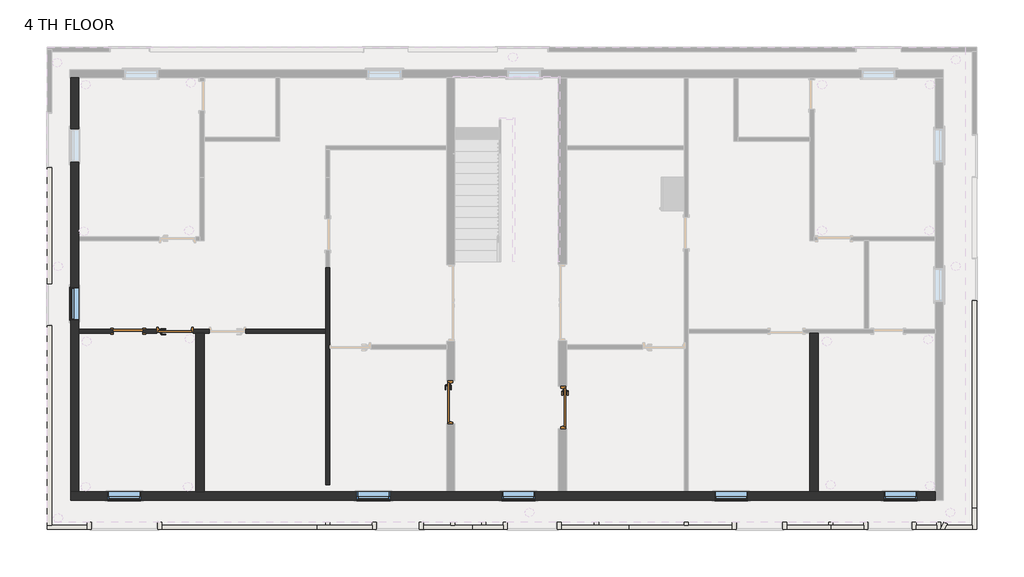
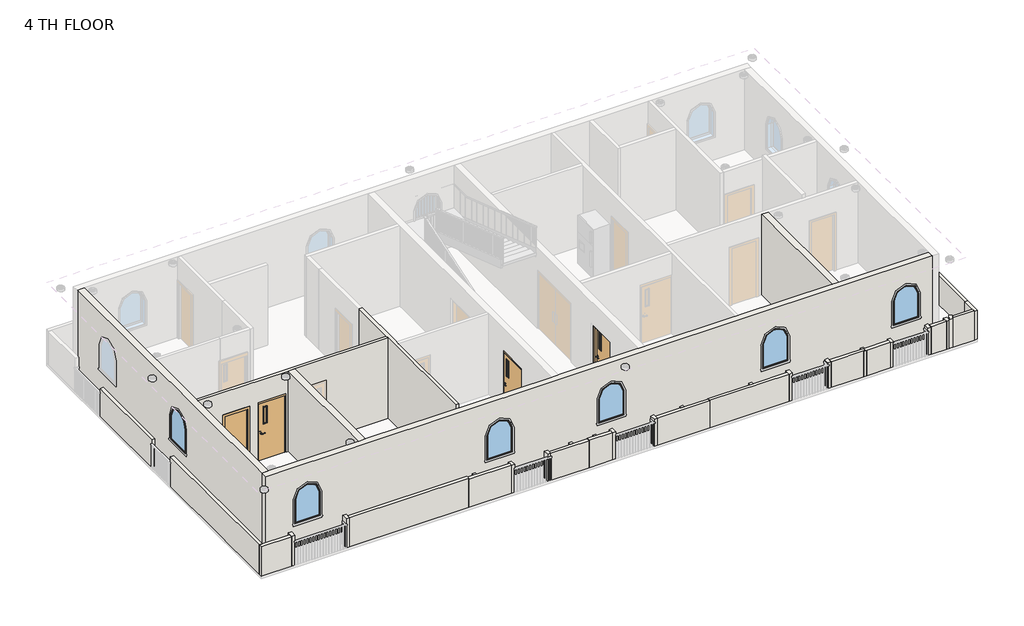
# One storey, part 1 of 7: 39 walls, 6 windows, 4 doors.
# Revit data of these elements (continued)
# Element 4 (IfcDoor, "Single-Flush : 2'8\"x 7'") (continued)
#   Phase Created = New Construction
#   Materials on its faces: "Door - Frame", "Door - Panel"
# Elements 5, 6 (IfcWall, "Generic - 4.5\"")
#   Top Offset = -0' - 6"
#   Base Offset = 0' - 0"
#   wall height = 10' - 0"
#   Phase Created = New Construction
#   Base Constraint = 4 TH FLOOR
#   Top Constraint = 5TH FLOOR
#   Materials on its faces: "Default Wall"
# Element 7 (IfcWall, "Generic - 4.5\"")
#   Top Offset = -6' - 10.1834"
#   Base Offset = 0' - 0"
#   wall height = 3' - 7.8166"
#   Phase Created = New Construction
#   Base Constraint = 4 TH FLOOR
#   Top Constraint = 5TH FLOOR
#   Materials on its faces: "Default Wall"
# Element 8 (IfcWall, "Generic - 4.5\"")
#   Top Offset = 0' - 0"
#   Base Offset = 0' - 0"
#   Unconnected Height = 3' - 8.64293"
#   wall height = 3' - 8.64293"
#   Phase Created = New Construction
#   Base Constraint = 4 TH FLOOR
#   Materials on its faces: "Default Wall"
# Element 9 (IfcWall, "Generic - 4.5\"")
#   Top Offset = -6' - 10.57009"
#   Base Offset = 0' - 0"
#   wall height = 3' - 7.42991"
#   Phase Created = New Construction
#   Base Constraint = 4 TH FLOOR
#   Top Constraint = 5TH FLOOR
#   Materials on its faces: "Default Wall"
# Element 10 (IfcWall, "Generic - 4.5\"")
#   Top Offset = -6' - 11.10495"
#   Base Offset = 0' - 0"
#   wall height = 3' - 6.89505"
#   Phase Created = New Construction
#   Base Constraint = 4 TH FLOOR
#   Top Constraint = 5TH FLOOR
#   Materials on its faces: "Default Wall"
# Element 11 (IfcWall, "Generic - 4.5\"")
#   Top Offset = -6' - 11.01332"
#   Base Offset = 0' - 0"
#   wall height = 3' - 6.98668"
#   Phase Created = New Construction
#   Base Constraint = 4 TH FLOOR
#   Top Constraint = 5TH FLOOR
#   Materials on its faces: "Default Wall"
# Element 12 (IfcWall, "Generic - 4.5\"")
#   Top Offset = -7' - 0.14651"
#   Base Offset = 0' - 0"
#   wall height = 3' - 5.85349"
#   Phase Created = New Construction
#   Base Constraint = 4 TH FLOOR
#   Top Constraint = 5TH FLOOR
#   Materials on its faces: "Default Wall"
# Element 13 (IfcWall, "Generic - 4.5\"")
#   Top Offset = -6' - 11.98199"
#   Base Offset = 0' - 0"
#   wall height = 3' - 6.01801"
#   Phase Created = New Construction
#   Base Constraint = 4 TH FLOOR
#   Top Constraint = 5TH FLOOR
#   Materials on its faces: "Default Wall"
# Elements 14, 16 (IfcWall, "Generic - 4.5\"")
#   Top Offset = -7' - 2"
#   Base Offset = 0' - 0"
#   wall height = 3' - 4"
#   Phase Created = New Construction
#   Base Constraint = 4 TH FLOOR
#   Top Constraint = 5TH FLOOR
#   Materials on its faces: "Default Wall"
# Element 15 (IfcWall, "Generic - 4.5\"")
#   Top Offset = -7' - 1.47546"
#   Base Offset = 0' - 0"
#   wall height = 3' - 4.52454"
#   Phase Created = New Construction
#   Base Constraint = 4 TH FLOOR
#   Top Constraint = 5TH FLOOR
#   Materials on its faces: "Default Wall"
# Elements 17, 33, 34 (IfcWall, "Generic - 4.5\"")
#   Top Offset = -7' - 2.10925"
#   Base Offset = 0' - 0"
#   wall height = 3' - 3.89075"
#   Phase Created = New Construction
#   Base Constraint = 4 TH FLOOR
#   Top Constraint = 5TH FLOOR
#   Materials on its faces: "Default Wall"
# Elements 18, 19 (IfcWall, "Generic - 4.5\"")
#   Top Offset = -7' - 1.54885"
#   Base Offset = 0' - 0"
#   wall height = 3' - 4.45115"
#   Phase Created = New Construction
#   Base Constraint = 4 TH FLOOR
#   Top Constraint = 5TH FLOOR
#   Materials on its faces: "Default Wall"
# Element 20 (IfcWall, "Generic - 4.5\"")
#   Top Offset = -7' - 1.35503"
#   Base Offset = 0' - 0"
#   wall height = 3' - 4.64497"
#   Phase Created = New Construction
#   Base Constraint = 4 TH FLOOR
#   Top Constraint = 5TH FLOOR
#   Materials on its faces: "Default Wall"
# Element 21 (IfcWall, "Generic - 4.5\"")
#   Top Offset = -7' - 3.70017"
#   Base Offset = 0' - 0"
#   wall height = 3' - 2.29983"
#   Phase Created = New Construction
#   Base Constraint = 4 TH FLOOR
#   Top Constraint = 5TH FLOOR
#   Materials on its faces: "Default Wall"
# Element 22 (IfcWall, "Generic - 4.5\"")
#   Top Offset = -7' - 3.69456"
#   Base Offset = 0' - 0"
#   wall height = 3' - 2.30544"
#   Phase Created = New Construction
#   Base Constraint = 4 TH FLOOR
#   Top Constraint = 5TH FLOOR
#   Materials on its faces: "Default Wall"
# Element 23 (IfcWall, "Generic - 4.5\"")
#   Top Offset = -7' - 4.34583"
#   Base Offset = 0' - 0"
#   wall height = 3' - 1.65417"
#   Phase Created = New Construction
#   Base Constraint = 4 TH FLOOR
#   Top Constraint = 5TH FLOOR
#   Materials on its faces: "Default Wall"
# Element 24 (IfcWall, "Generic - 4.5\"")
#   Top Offset = -7' - 3.82361"
#   Base Offset = 0' - 0"
#   wall height = 3' - 2.17639"
#   Phase Created = New Construction
#   Base Constraint = 4 TH FLOOR
#   Top Constraint = 5TH FLOOR
#   Materials on its faces: "Default Wall"
# Element 25 (IfcWall, "Generic - 4.5\"")
#   Top Offset = -7' - 4.51157"
#   Base Offset = 0' - 0"
#   wall height = 3' - 1.48843"
#   Phase Created = New Construction
#   Base Constraint = 4 TH FLOOR
#   Top Constraint = 5TH FLOOR
#   Materials on its faces: "Default Wall"
# Element 26 (IfcWall, "Generic - 4.5\"")
#   Top Offset = -7' - 1.5942"
#   Base Offset = 0' - 0"
#   wall height = 3' - 4.4058"
#   Phase Created = New Construction
#   Base Constraint = 4 TH FLOOR
#   Top Constraint = 5TH FLOOR
#   Materials on its faces: "Default Wall"
# Elements 27, 28 (IfcWall, "Generic - 4.5\"")
#   Top Offset = -7' - 0.71294"
#   Base Offset = 0' - 0"
#   wall height = 3' - 5.28706"
#   Phase Created = New Construction
#   Base Constraint = 4 TH FLOOR
#   Top Constraint = 5TH FLOOR
#   Materials on its faces: "Default Wall"
# Element 29 (IfcWall, "Generic - 4.5\"")
#   Top Offset = -7' - 0.30229"
#   Base Offset = 0' - 0"
#   wall height = 3' - 5.69771"
#   Phase Created = New Construction
#   Base Constraint = 4 TH FLOOR
#   Top Constraint = 5TH FLOOR
#   Materials on its faces: "Default Wall"
# Element 30 (IfcWall, "Generic - 4.5\"")
#   Top Offset = -7' - 1.97028"
#   Base Offset = 0' - 0"
#   wall height = 3' - 4.02972"
#   Phase Created = New Construction
#   Base Constraint = 4 TH FLOOR
#   Top Constraint = 5TH FLOOR
#   Materials on its faces: "Default Wall"
# Element 31 (IfcWall, "Generic - 4.5\"")
#   Top Offset = -7' - 1.40393"
#   Base Offset = 0' - 0"
#   wall height = 3' - 4.59607"
#   Phase Created = New Construction
#   Base Constraint = 4 TH FLOOR
#   Top Constraint = 5TH FLOOR
#   Materials on its faces: "Default Wall"
# Element 32 (IfcWall, "Generic - 4.5\"")
#   Top Offset = -7' - 1.68978"
#   Base Offset = 0' - 0"
#   wall height = 3' - 4.31022"
#   Phase Created = New Construction
#   Base Constraint = 4 TH FLOOR
#   Top Constraint = 5TH FLOOR
#   Materials on its faces: "Default Wall"
# Elements 35, 36 (IfcWall, "Generic - 4.5\"")
#   Top Offset = -6' - 10.38959"
#   Base Offset = 0' - 0"
#   wall height = 3' - 7.61041"
#   Phase Created = New Construction
#   Base Constraint = 4 TH FLOOR
#   Top Constraint = 5TH FLOOR
#   Materials on its faces: "Default Wall"
# Element 37 (IfcWall, "Generic - 4.5\"")
#   Top Offset = 0' - 0"
#   Base Offset = 0' - 0"
#   Unconnected Height = 3' - 7.86488"
#   wall height = 3' - 7.86488"
#   Phase Created = New Construction
#   Base Constraint = 4 TH FLOOR
#   Materials on its faces: "Default Wall"
# Element 38 (IfcWall, "Generic - 4.5\"")
#   Top Offset = -7' - 0.76215"
#   Base Offset = 0' - 0"
#   wall height = 3' - 5.23785"
#   Phase Created = New Construction
#   Base Constraint = 4 TH FLOOR
#   Top Constraint = 5TH FLOOR
#   Materials on its faces: "Default Wall"
# Element 39 (IfcWall, "Generic - 4.5\"")
#   Top Offset = -6' - 11.21767"
#   Base Offset = 0' - 0"
#   wall height = 3' - 6.78233"
#   Phase Created = New Construction
#   Base Constraint = 4 TH FLOOR
#   Top Constraint = 5TH FLOOR
#   Materials on its faces: "Default Wall"
# Elements 40, 41, 42, 43 (IfcWall, "Generic - 9\"")
#   Top Offset = -0' - 6"
#   Base Offset = 0' - 0"
#   wall height = 10' - 0"
#   Phase Created = New Construction
#   Base Constraint = 4 TH FLOOR
#   Top Constraint = 5TH FLOOR
#   Materials on its faces: "Concrete Masonry Units"
# Element 44 (IfcWindow, "Window-Fixed-Round-Top : 3' x 4'")
#   Mark = "171"
#   Window Inset = 0' - 0"
#   Interior Wall Closure = 0' - 2 1/4"
#   Frame Extension = 0' - 0 1/4"
#   Exterior Wall Closure = 0' - 1 1/4"
#   Interior Trim Visibility = yes
#   Exterior Trim Visibility = yes
#   Phase Created = New Construction
#   Materials on its faces: "Wood - Stained", "Clad - White", "Glass"
# Element 45 (IfcWindow, "Window-Fixed-Round-Top : 3' x 4'")
#   Mark = "172"
#   Window Inset = 0' - 0"
#   Interior Wall Closure = 0' - 2 1/4"
#   Frame Extension = 0' - 0 1/4"
#   Exterior Wall Closure = 0' - 1 1/4"
#   Interior Trim Visibility = yes
#   Exterior Trim Visibility = yes
#   Phase Created = New Construction
#   Materials on its faces: "Wood - Stained", "Clad - White", "Glass"
# Element 46 (IfcWindow, "Window-Fixed-Round-Top : 3' x 4'")
#   Mark = "173"
#   Window Inset = 0' - 0"
#   Interior Wall Closure = 0' - 2 1/4"
#   Frame Extension = 0' - 0 1/4"
#   Exterior Wall Closure = 0' - 1 1/4"
#   Interior Trim Visibility = yes
#   Exterior Trim Visibility = yes
#   Phase Created = New Construction
#   Materials on its faces: "Wood - Stained", "Clad - White", "Glass"
# Element 47 (IfcWindow, "Window-Fixed-Round-Top : 3' x 4'")
#   Mark = "174"
#   Window Inset = 0' - 0"
#   Interior Wall Closure = 0' - 2 1/4"
#   Frame Extension = 0' - 0 1/4"
#   Exterior Wall Closure = 0' - 1 1/4"
#   Interior Trim Visibility = yes
#   Exterior Trim Visibility = yes
#   Phase Created = New Construction
#   Materials on its faces: "Wood - Stained", "Clad - White", "Glass"
# Element 48 (IfcWindow, "Window-Fixed-Round-Top : 3' x 4'")
#   Mark = "175"
#   Window Inset = 0' - 0"
#   Interior Wall Closure = 0' - 2 1/4"
#   Frame Extension = 0' - 0 1/4"
#   Exterior Wall Closure = 0' - 1 1/4"
#   Interior Trim Visibility = yes
#   Exterior Trim Visibility = yes
#   Phase Created = New Construction
#   Materials on its faces: "Wood - Stained", "Clad - White", "Glass"
# Element 49 (IfcWindow, "Window-Fixed-Round-Top : 3' x 4'")
#   Mark = "183"
#   Window Inset = 0' - 0"
#   Interior Wall Closure = 0' - 2 1/4"
#   Frame Extension = 0' - 0 1/4"
#   Exterior Wall Closure = 0' - 1 1/4"
#   Interior Trim Visibility = yes
#   Exterior Trim Visibility = yes
#   Phase Created = New Construction
#   Materials on its faces: "Wood - Stained", "Clad - White", "Glass"
# Materials
#   "Wood - Birch": class "Wood", colour RGB 166 116 52, transparency 0, Cost = 0
#   "Glass": class "Glass", colour RGB 0 128 192, transparency 0.75, Description = "Soda Lime Glass", Cost = 0
#   "Metal - Paint Finish - Grey": class "Paint", colour RGB 104 104 104, transparency 0, Cost = 0
#   "Aluminum": class "Metal", colour RGB 247 247 247, transparency 0, Description = "Aluminum 6061", Cost = 0
#   "Door - Panel": class "Wood", colour RGB 210 159 95, transparency 0, Cost = 0
#   "Door - Frame": colour RGB 118 70 51, transparency 0, Cost = 0
#   "Concrete Masonry Units": class "Masonry", colour RGB 227 227 227, transparency 0, Description = "Concrete masonry units", Cost = 0
#   "Wood - Stained": class "Wood", colour RGB 224 178 126, transparency 0, Cost = 0
#   "Clad - White": class "Wood", colour RGB 242 242 238, transparency 0, Cost = 0
#   "Default Wall": colour RGB 128 128 128, transparency 0, Cost = 0
